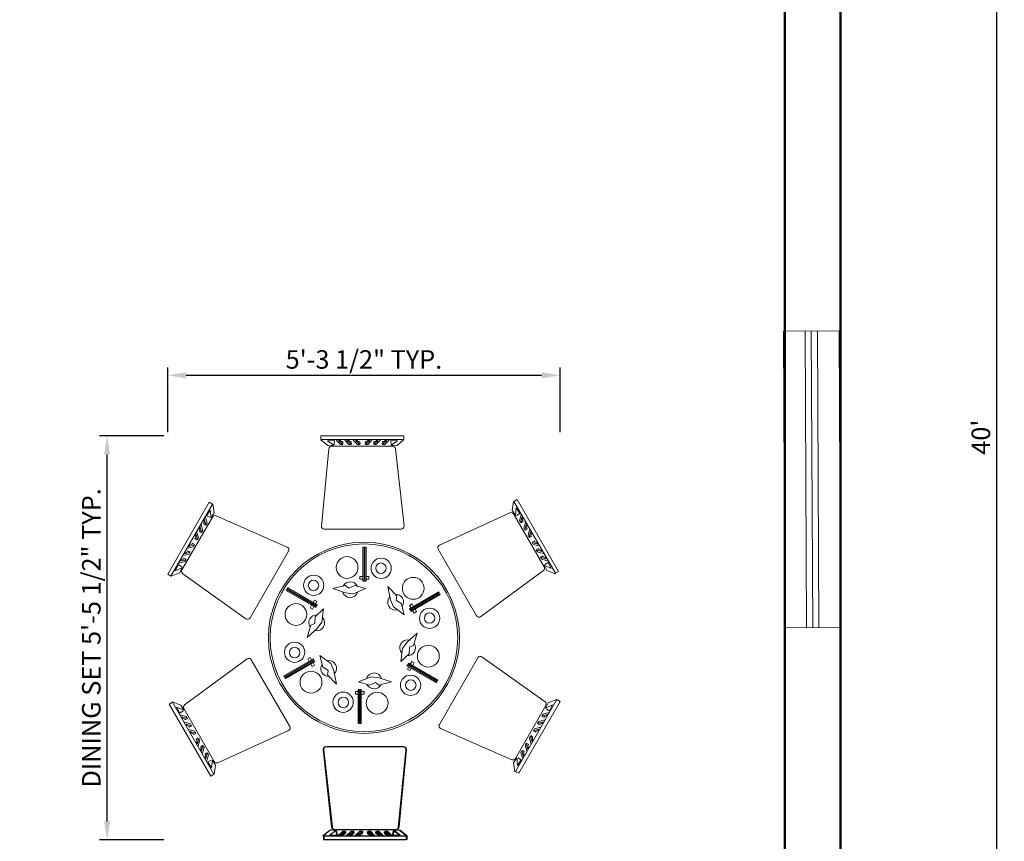
# Model space of a CAD drawing. Units: inches. Extents: x 108 to 1546, y -229 to 513.
# Tile 6 of 11: x 910 to 1070, y 171 to 304. Entities that reach past the tile are written whole.
import ezdxf

# ---------------------------------------------------------------- set-up
doc = ezdxf.new("R2010")
doc.units = ezdxf.units.IN
for name, color, linetype, lineweight in [('A-ANNO-DIMS', 2, 'Continuous', 18), ('A-FURN', 8, 'Continuous', 13), ('wall', 7, 'Continuous', 50), ('WINDOW', 212, 'Continuous', 18)]:
    doc.layers.add(name, color=color, linetype=linetype, lineweight=lineweight)
doc.styles.get("Standard").update_dxf_attribs({"font": 'arial.ttf'})
doc.dimstyles.new('ISO-25', dxfattribs={"dimtxt": 3, "dimasz": 3, "dimexe": 1.25, "dimexo": 0.625, "dimtad": 1, "dimdec": 1, "dimlunit": 3, "dimtxsty": 'Standard', "dimcen": 2.5, "dimadec": 0, "dimazin": 0, "dimtfac": 1, "dimtdec": 1, "dimtmove": 0, "dimatfit": 3, "dimfxl": 1, "dimarcsym": 0})

# ---------------------------------------------------------------- blocks, each defined once
blk = doc.blocks.new('A$C45501D90')
for p, q in [((-242.2, 1133.5), (224, 1133.5)), ((-242.2, 1112.8), (-242.2, 1133.5)), ((224, 1112.8), (-242.2, 1112.8)), ((-242.2, 1111.2), (-202.3, 1079.2)), ((-203.9, 1106.4), (-165.6, 1108)), ((-165.6, 1108), (-167.2, 1085.6)), ((-156, 1109.6), (-132, 1085.6)), ((-119.3, 1085.6), (-143.2, 1108)), ((-143.2, 1108), (-133.6, 1108)), ((-133.6, 1108), (-122.5, 1098.4)), ((-108.1, 1109.6), (-84.1, 1085.6)), ((-71.4, 1085.6), (-95.3, 1108)), ((-95.3, 1108), (-85.7, 1108)), ((-85.7, 1108), (-74.6, 1098.4)), ((-60.2, 1109.6), (-36.2, 1085.6)), ((-23.5, 1085.6), (-47.4, 1108)), ((-47.4, 1108), (-37.8, 1108)), ((-37.8, 1108), (-26.7, 1098.4)), ((8.5, 1085.6), (32.4, 1108)), ((22.8, 1108), (11.6, 1098.4)), ((45.2, 1109.6), (21.2, 1085.6)), ((32.4, 1108), (22.8, 1108)), ((56.3, 1085.6), (80.3, 1108)), ((70.7, 1108), (59.5, 1098.4)), ((93.1, 1109.6), (69.1, 1085.6)), ((80.3, 1108), (70.7, 1108)), ((104.2, 1085.6), (128.2, 1108)), ((118.6, 1108), (107.4, 1098.4)), ((141, 1109.6), (117, 1085.6)), ((128.2, 1108), (118.6, 1108)), ((188.9, 1106.4), (150.5, 1108)), ((150.5, 1108), (152.1, 1085.6)), ((224, 1112.8), (187.3, 1079.2)), ((224, 1133.5), (224, 1112.8)), ((-197.3, 1061.6), (-238.9, 627.6)), ((-168.8, 1080.8), (-203.9, 1106.4)), ((-202.3, 1079.2), (-168.8, 1080.8)), ((161.8, 1076.1), (-181.4, 1076.1)), ((-132, 1085.6), (-119.3, 1085.6)), ((-122.5, 1098.4), (-119.3, 1101.6)), ((-119.3, 1101.6), (-117.7, 1087.2)), ((-84.1, 1085.6), (-71.4, 1085.6)), ((-74.6, 1098.4), (-71.4, 1101.6)), ((-71.4, 1101.6), (-69.8, 1087.2)), ((-36.2, 1085.6), (-23.5, 1085.6)), ((-26.7, 1098.4), (-23.5, 1101.6)), ((-23.5, 1101.6), (-21.9, 1087.2)), ((8.5, 1101.6), (6.9, 1087.2)), ((11.6, 1098.4), (8.5, 1101.6)), ((21.2, 1085.6), (8.5, 1085.6)), ((56.3, 1101.6), (54.8, 1087.2)), ((59.5, 1098.4), (56.3, 1101.6)), ((69.1, 1085.6), (56.3, 1085.6)), ((104.2, 1101.6), (102.6, 1087.2)), ((107.4, 1098.4), (104.2, 1101.6)), ((117, 1085.6), (104.2, 1085.6)), ((153.7, 1080.8), (188.9, 1106.4)), ((187.3, 1079.2), (153.7, 1080.8)), ((225.2, 627.8), (177.6, 1061.8)), ((842.6, 766.1), (860.5, 776.5)), ((860.5, 776.5), (1093.6, 372.8)), ((-1102.7, 357), (-869.7, 760.7)), ((-851.7, 750.4), (-1084.8, 346.6)), ((-869.7, 760.7), (-851.7, 750.4)), ((-848.7, 752.3), (-841, 701.8)), ((841.2, 765.3), (833.5, 714.8)), ((1075.7, 362.4), (842.6, 766.1)), ((851.7, 686.6), (856.2, 729.8)), ((856.2, 729.8), (876.7, 697.4)), ((-851, 678.1), (-1022.6, 380.9)), ((-895.4, 665), (-900.2, 656.7)), ((-888.1, 633.1), (-895.4, 665)), ((-890.4, 676.9), (-881.7, 644.2)), ((-863.7, 716.7), (-884.3, 684.4)), ((-884.3, 684.4), (-864.1, 674.6)), ((-859.2, 673.6), (-863.7, 716.7)), ((-841, 701.8), (-859.2, 673.6)), ((-431.1, 509), (-830.8, 684.8)), ((820.7, 701.7), (424.1, 520.7)), ((833.5, 714.8), (851.7, 686.6)), ((1012.8, 397.9), (841.2, 695.1)), ((876.7, 697.4), (856.6, 687.6)), ((882.9, 689.9), (874.2, 657.2)), ((880.6, 646.1), (887.9, 678)), ((887.9, 678), (892.7, 669.7)), ((892.7, 669.7), (890, 655.2)), ((-919.4, 623.5), (-924.2, 615.2)), ((-924.2, 615.2), (-921.5, 600.8)), ((-912, 591.6), (-919.4, 623.5)), ((-914.4, 635.4), (-905.6, 602.7)), ((-897.5, 642.2), (-901.9, 641.1)), ((-901.9, 641.1), (-890.2, 632.5)), ((-900.2, 656.7), (-897.5, 642.2)), ((-881.7, 644.2), (-888.1, 633.1)), ((-223, 610.1), (209.4, 610.1)), ((874.2, 657.2), (880.6, 646.1)), ((894.4, 654.1), (882.7, 645.5)), ((890, 655.2), (894.4, 654.1)), ((906.9, 648.4), (898.1, 615.7)), ((898.1, 615.7), (904.5, 604.6)), ((904.5, 604.6), (911.9, 636.5)), ((918.3, 612.6), (906.7, 604)), ((911.9, 636.5), (916.7, 628.2)), ((916.7, 628.2), (914, 613.8)), ((914, 613.8), (918.3, 612.6)), ((-945.4, 559.3), (-949.8, 558.1)), ((-949.8, 558.1), (-938.1, 549.6)), ((-943.3, 582), (-948.1, 573.8)), ((-948.1, 573.8), (-945.4, 559.3)), ((-936, 550.1), (-943.3, 582)), ((-938.3, 593.9), (-929.6, 561.2)), ((-929.6, 561.2), (-936, 550.1)), ((-921.5, 600.8), (-925.8, 599.6)), ((-925.8, 599.6), (-914.2, 591)), ((-905.6, 602.7), (-912, 591.6)), ((930.8, 606.9), (922.1, 574.2)), ((922.1, 574.2), (928.4, 563.1)), ((928.4, 563.1), (935.8, 595.1)), ((942.3, 571.1), (930.6, 562.6)), ((935.8, 595.1), (940.6, 586.8)), ((940.6, 586.8), (937.9, 572.3)), ((937.9, 572.3), (942.3, 571.1)), ((-991, 502.7), (-958.3, 511.4)), ((-951.9, 522.5), (-983.2, 512.9)), ((-983.2, 512.9), (-978.5, 521.2)), ((-978.5, 521.2), (-964.6, 526.1)), ((-964.6, 526.1), (-965.7, 530.5)), ((-965.7, 530.5), (-952.5, 524.7)), ((-958.3, 511.4), (-951.9, 522.5)), ((-5.6, 508.7, 90.8), (0.4, 508.7, 90.8)), ((-5.6, 317.7, 90.8), (-5.6, 508.7, 90.8)), ((0.4, 508.7, 90.8), (0.4, 317.7, 90.8)), ((5.8, 317.7, 90.8), (5.8, 508.7, 90.8)), ((5.8, 508.7, 90.8), (11.8, 508.7, 90.8)), ((11.8, 508.7, 90.8), (11.8, 317.7, 90.8)), ((416.9, 498.2), (633.1, 123.7)), ((950.8, 524.4), (944.4, 535.5)), ((944.4, 535.5), (975.7, 525.9)), ((958.2, 543.5), (945, 537.7)), ((983.5, 515.7), (950.8, 524.4)), ((957.1, 539.1), (958.2, 543.5)), ((970.9, 534.2), (957.1, 539.1)), ((982.2, 502), (968.9, 496.2)), ((975.7, 525.9), (970.9, 534.2)), ((981, 497.6), (982.2, 502)), ((-1026.3, 438.3), (-1012.5, 443.1)), ((-1015, 461.2), (-982.3, 469.9)), ((-1012.5, 443.1), (-1013.6, 447.5)), ((-1013.6, 447.5), (-1000.4, 441.7)), ((-975.9, 481), (-1007.2, 471.4)), ((-1007.2, 471.4), (-1002.4, 479.7)), ((-1002.4, 479.7), (-988.5, 484.6)), ((-988.5, 484.6), (-989.7, 489)), ((-989.7, 489), (-976.5, 483.2)), ((-982.3, 469.9), (-975.9, 481)), ((-639.9, 111.9), (-423.7, 486.4)), ((968.4, 494), (999.7, 484.4)), ((974.7, 483), (968.4, 494)), ((1007.4, 474.2), (974.7, 483)), ((994.9, 492.7), (981, 497.6)), ((998.7, 441.5), (992.3, 452.5)), ((992.3, 452.5), (1023.6, 443)), ((1006.1, 460.5), (992.9, 454.7)), ((999.7, 484.4), (994.9, 492.7)), ((1005, 456.2), (1006.1, 460.5)), ((1018.8, 451.3), (1005, 456.2)), ((1023.6, 443), (1018.8, 451.3)), ((-1060.1, 376.6), (-1042.3, 410.6)), ((-1020.4, 394.3), (-1060.1, 376.6)), ((-1042.3, 410.6), (-1023.8, 398.1)), ((-1038.9, 419.7), (-1006.2, 428.5)), ((-1035.8, 364.4), (-1020.4, 394.3)), ((-999.8, 439.5), (-1031.1, 430)), ((-1031.1, 430), (-1026.3, 438.3)), ((-1006.2, 428.5), (-999.8, 439.5)), ((1031.4, 432.7), (998.7, 441.5)), ((1028.3, 377.5), (1012.9, 407.3)), ((1012.9, 407.3), (1052.6, 389.6)), ((1034.8, 423.6), (1016.3, 411.1)), ((1052.6, 389.6), (1034.8, 423.6)), ((-1084.8, 346.6), (-1102.7, 357)), ((-1083.4, 345.8), (-1035.8, 364.4)), ((-1018, 360), (-663, 106.9)), ((-22.3, 329.1, 90.8), (-22.3, 344.6, 90.8)), ((-22.3, 344.6, 90.8), (-5.6, 344.6, 90.8)), ((0.4, 344.6, 90.8), (5.8, 344.6, 90.8)), ((11.8, 344.6, 90.8), (27.3, 344.6, 90.8)), ((27.3, 344.6, 90.8), (27.3, 329.1, 90.8)), ((656.3, 118.9), (1008.4, 377.1)), ((1075.9, 358.8), (1028.3, 377.5)), ((1093.6, 372.8), (1075.7, 362.4)), ((-430.6, 275.2, 90.8), (-427.6, 280.3, 90.8)), ((-427.6, 280.3, 90.8), (-262.3, 184.9, 90.8)), ((-175.3, 276.1, 90.8), (-104.8, 293.2, 90.8)), ((-104.8, 293.2, 90.8), (-85.5, 278.4, 90.8)), ((-85.5, 278.4, 90.8), (-52.1, 293.9, 90.8)), ((-52.1, 293.9, 90.8), (9.5, 276.1, 90.8)), ((-5.6, 329.1, 90.8), (-22.3, 329.1, 90.8)), ((0.4, 317.7, 90.8), (-5.6, 317.7, 90.8)), ((5.8, 329.1, 90.8), (0.4, 329.1, 90.8)), ((11.8, 317.7, 90.8), (5.8, 317.7, 90.8)), ((27.3, 329.1, 90.8), (11.8, 329.1, 90.8)), ((134.3, 288, 90.8), (184.3, 235.5, 90.8)), ((149.7, 213.9, 90.8), (134.3, 288, 90.8)), ((-436.3, 265.3, 90.8), (-433.3, 270.5, 90.8)), ((-270.9, 169.9, 90.8), (-436.3, 265.3, 90.8)), ((-433.3, 270.5, 90.8), (-267.9, 175, 90.8)), ((-265.2, 179.7, 90.8), (-430.6, 275.2, 90.8)), ((-103.3, 252.4, 90.8), (-175.3, 276.1, 90.8)), ((-59.5, 246.5, 90.8), (-103.3, 252.4, 90.8)), ((9.5, 276.1, 90.8), (-59.5, 246.5, 90.8)), ((184.3, 235.5, 90.8), (181.1, 211.4, 90.8)), ((255.2, 161.9, 90.8), (420.6, 257.3, 90.8)), ((423.5, 252.2, 90.8), (258.2, 156.7, 90.8)), ((260.9, 152, 90.8), (426.2, 247.5, 90.8)), ((429.2, 242.3, 90.8), (263.8, 146.9, 90.8)), ((420.6, 257.3, 90.8), (423.5, 252.2, 90.8)), ((426.2, 247.5, 90.8), (429.2, 242.3, 90.8)), ((-302.5, 168.8, 90.8), (-294.2, 183.3, 90.8)), ((-289.1, 161.1, 90.8), (-302.5, 168.8, 90.8)), ((-291.2, 188.5, 90.8), (-288.5, 193.1, 90.8)), ((-280.7, 175.5, 90.8), (-289.1, 161.1, 90.8)), ((-285.5, 198.3, 90.8), (-277.8, 211.7, 90.8)), ((-277.8, 211.7, 90.8), (-264.3, 204, 90.8)), ((-275.1, 185.4, 90.8), (-277.8, 180.7, 90.8)), ((-264.3, 204, 90.8), (-272.1, 190.5, 90.8)), ((-267.9, 175, 90.8), (-270.9, 169.9, 90.8)), ((-262.3, 184.9, 90.8), (-265.2, 179.7, 90.8)), ((166.5, 173, 90.8), (149.7, 213.9, 90.8)), ((226.7, 128.1, 90.8), (166.5, 173, 90.8)), ((181.1, 211.4, 90.8), (211.3, 190.3, 90.8)), ((211.3, 190.3, 90.8), (226.7, 128.1, 90.8)), ((256.6, 182, 90.8), (270.1, 189.8, 90.8)), ((265, 167.5, 90.8), (256.6, 182, 90.8)), ((270.1, 189.8, 90.8), (278.4, 175.3, 90.8)), ((281.4, 170.1, 90.8), (284.1, 165.5, 90.8)), ((-276.8, 80.9, 90.8), (-273.6, 117.6, 90.8)), ((-273.6, 117.6, 90.8), (-227.4, 162.1, 90.8)), ((-227.4, 162.1, 90.8), (-236.2, 87.5, 90.8)), ((258.2, 156.7, 90.8), (255.2, 161.9, 90.8)), ((263.8, 146.9, 90.8), (260.9, 152, 90.8)), ((270.7, 157.7, 90.8), (268, 162.4, 90.8)), ((281.4, 139.1, 90.8), (273.7, 152.5, 90.8)), ((294.9, 146.8, 90.8), (281.4, 139.1, 90.8)), ((287.1, 160.3, 90.8), (294.9, 146.8, 90.8)), ((-319.8, 2.1, 90.8), (-299.3, 71.7, 90.8)), ((-299.3, 71.7, 90.8), (-276.8, 80.9, 90.8)), ((-236.2, 87.5, 90.8), (-263.2, 52.5, 90.8)), ((-263.2, 52.5, 90.8), (-319.8, 2.1, 90.8)), ((242.9, -24.6, 90.8), (299.4, 25.9, 90.8)), ((299.4, 25.9, 90.8), (278.9, -43.7, 90.8)), ((215.8, -59.5, 90.8), (242.9, -24.6, 90.8)), ((256.4, -53, 90.8), (253.2, -89.7, 90.8)), ((278.9, -43.7, 90.8), (256.4, -53, 90.8)), ((-247, -100.1, 90.8), (-186.8, -145, 90.8)), ((-231.7, -162.3, 90.8), (-247, -100.1, 90.8)), ((207, -134.1, 90.8), (215.8, -59.5, 90.8)), ((253.2, -89.7, 90.8), (207, -134.1, 90.8)), ((1018, -360), (663, -106.9)), ((-656.3, -118.9), (-1008.4, -377.1)), ((-416.9, -498.2), (-633.1, -123.7)), ((-449.6, -214.4, 90.8), (-284.2, -118.9, 90.8)), ((-281.2, -124.1, 90.8), (-446.6, -219.5, 90.8)), ((-443.9, -224.2, 90.8), (-278.5, -128.7, 90.8)), ((-275.5, -133.9, 90.8), (-440.9, -229.4, 90.8)), ((-315.2, -118.9, 90.8), (-301.8, -111.1, 90.8)), ((-307.5, -132.3, 90.8), (-315.2, -118.9, 90.8)), ((-301.8, -142.1, 90.8), (-304.5, -137.5, 90.8)), ((-301.8, -111.1, 90.8), (-294, -124.6, 90.8)), ((-290.4, -161.8, 90.8), (-298.8, -147.3, 90.8)), ((-291, -129.7, 90.8), (-288.3, -134.4, 90.8)), ((-277, -154, 90.8), (-290.4, -161.8, 90.8)), ((-285.4, -139.5, 90.8), (-277, -154, 90.8)), ((-284.2, -118.9, 90.8), (-281.2, -124.1, 90.8)), ((-278.5, -128.7, 90.8), (-275.5, -133.9, 90.8)), ((-201.5, -183.4, 90.8), (-231.7, -162.3, 90.8)), ((-186.8, -145, 90.8), (-170.1, -185.9, 90.8)), ((241.9, -156.9, 90.8), (244.9, -151.7, 90.8)), ((407.3, -252.4, 90.8), (241.9, -156.9, 90.8)), ((244, -176, 90.8), (251.7, -162.5, 90.8)), ((244.9, -151.7, 90.8), (410.3, -247.2, 90.8)), ((247.6, -147.1, 90.8), (250.6, -141.9, 90.8)), ((413, -242.5, 90.8), (247.6, -147.1, 90.8)), ((250.6, -141.9, 90.8), (415.9, -237.4, 90.8)), ((254.7, -157.4, 90.8), (257.4, -152.7, 90.8)), ((260.4, -147.6, 90.8), (268.7, -133.1, 90.8)), ((270.8, -160.5, 90.8), (268.1, -165.1, 90.8)), ((268.7, -133.1, 90.8), (282.2, -140.8, 90.8)), ((282.2, -140.8, 90.8), (273.8, -155.3, 90.8)), ((639.9, -111.9), (423.7, -486.4)), ((-446.6, -219.5, 90.8), (-449.6, -214.4, 90.8)), ((-204.7, -207.6, 90.8), (-201.5, -183.4, 90.8)), ((-154.7, -260.1, 90.8), (-204.7, -207.6, 90.8)), ((-170.1, -185.9, 90.8), (-154.7, -260.1, 90.8)), ((-29.8, -248.2, 90.8), (39.2, -218.5, 90.8)), ((39.2, -218.5, 90.8), (83, -224.4, 90.8)), ((257.4, -183.7, 90.8), (244, -176, 90.8)), ((265.2, -170.3, 90.8), (257.4, -183.7, 90.8)), ((-440.9, -229.4, 90.8), (-443.9, -224.2, 90.8)), ((31.8, -266, 90.8), (-29.8, -248.2, 90.8)), ((65.2, -250.4, 90.8), (31.8, -266, 90.8)), ((84.4, -265.2, 90.8), (65.2, -250.4, 90.8)), ((83, -224.4, 90.8), (154.9, -248.2, 90.8)), ((154.9, -248.2, 90.8), (84.4, -265.2, 90.8)), ((410.3, -247.2, 90.8), (407.3, -252.4, 90.8)), ((415.9, -237.4, 90.8), (413, -242.5, 90.8)), ((-47.6, -316.6, 90.8), (-47.6, -301.1, 90.8)), ((-47.6, -301.1, 90.8), (-32.1, -301.1, 90.8)), ((-32.1, -316.6, 90.8), (-47.6, -316.6, 90.8)), ((-32.1, -480.7, 90.8), (-32.1, -289.8, 90.8)), ((-32.1, -289.8, 90.8), (-26.1, -289.8, 90.8)), ((-26.1, -289.8, 90.8), (-26.1, -480.7, 90.8)), ((-26.1, -301.1, 90.8), (-20.8, -301.1, 90.8)), ((-20.8, -316.6, 90.8), (-26.1, -316.6, 90.8)), ((-20.8, -480.7, 90.8), (-20.8, -289.8, 90.8)), ((-20.8, -289.8, 90.8), (-14.8, -289.8, 90.8)), ((-14.8, -289.8, 90.8), (-14.8, -480.7, 90.8)), ((-14.8, -301.1, 90.8), (1.9, -301.1, 90.8)), ((1.9, -316.6, 90.8), (-14.8, -316.6, 90.8)), ((1.9, -301.1, 90.8), (1.9, -316.6, 90.8)), ((-1093.6, -372.8), (-1075.7, -362.4)), ((-860.5, -776.5), (-1093.6, -372.8)), ((-1075.9, -358.8), (-1028.3, -377.5)), ((-1075.7, -362.4), (-842.6, -766.1)), ((-1028.3, -377.5), (-1012.9, -407.3)), ((851, -678.1), (1022.6, -380.9)), ((851.7, -750.4), (1084.8, -346.6)), ((1102.7, -357), (869.7, -760.7)), ((1035.8, -364.4), (1020.4, -394.3)), ((1020.4, -394.3), (1060.1, -376.6)), ((1083.4, -345.8), (1035.8, -364.4)), ((1060.1, -376.6), (1042.3, -410.6)), ((1084.8, -346.6), (1102.7, -357)), ((-1052.6, -389.6), (-1034.8, -423.6)), ((-1012.9, -407.3), (-1052.6, -389.6)), ((-1034.8, -423.6), (-1016.3, -411.1)), ((-1031.4, -432.7), (-998.7, -441.5)), ((-1012.8, -397.9), (-841.2, -695.1)), ((-998.7, -441.5), (-992.3, -452.5)), ((1006.2, -428.5), (999.8, -439.5)), ((999.8, -439.5), (1031.1, -430)), ((1013.6, -447.5), (1000.4, -441.7)), ((1038.9, -419.7), (1006.2, -428.5)), ((1026.3, -438.3), (1012.5, -443.1)), ((1042.3, -410.6), (1023.8, -398.1)), ((1031.1, -430), (1026.3, -438.3)), ((-1023.6, -443), (-1018.8, -451.3)), ((-992.3, -452.5), (-1023.6, -443)), ((-1018.8, -451.3), (-1005, -456.2)), ((-1007.4, -474.2), (-974.7, -483)), ((-1006.1, -460.5), (-992.9, -454.7)), ((-1005, -456.2), (-1006.1, -460.5)), ((-968.4, -494), (-999.7, -484.4)), ((-999.7, -484.4), (-994.9, -492.7)), ((-994.9, -492.7), (-981, -497.6)), ((-982.2, -502), (-968.9, -496.2)), ((-981, -497.6), (-982.2, -502)), ((-974.7, -483), (-968.4, -494)), ((-26.1, -480.7, 90.8), (-32.1, -480.7, 90.8)), ((-14.8, -480.7, 90.8), (-20.8, -480.7, 90.8)), ((982.3, -469.9), (975.9, -481)), ((975.9, -481), (1007.2, -471.4)), ((989.7, -489), (976.5, -483.2)), ((1015, -461.2), (982.3, -469.9)), ((1002.4, -479.7), (988.5, -484.6)), ((988.5, -484.6), (989.7, -489)), ((1007.2, -471.4), (1002.4, -479.7)), ((1012.5, -443.1), (1013.6, -447.5)), ((-983.5, -515.7), (-950.8, -524.4)), ((-944.4, -535.5), (-975.7, -525.9)), ((-975.7, -525.9), (-970.9, -534.2)), ((-970.9, -534.2), (-957.1, -539.1)), ((-958.2, -543.5), (-945, -537.7)), ((-957.1, -539.1), (-958.2, -543.5)), ((-950.8, -524.4), (-944.4, -535.5)), ((-820.7, -701.7), (-424.1, -520.7)), ((431.1, -509), (830.8, -684.8)), ((929.6, -561.2), (936, -550.1)), ((936, -550.1), (943.3, -582)), ((949.8, -558.1), (938.1, -549.6)), ((958.3, -511.4), (951.9, -522.5)), ((951.9, -522.5), (983.2, -512.9)), ((965.7, -530.5), (952.5, -524.7)), ((991, -502.7), (958.3, -511.4)), ((978.5, -521.2), (964.6, -526.1)), ((964.6, -526.1), (965.7, -530.5)), ((983.2, -512.9), (978.5, -521.2)), ((-942.3, -571.1), (-930.6, -562.6)), ((-937.9, -572.3), (-942.3, -571.1)), ((-940.6, -586.8), (-937.9, -572.3)), ((-935.8, -595.1), (-940.6, -586.8)), ((-928.4, -563.1), (-935.8, -595.1)), ((-930.8, -606.9), (-922.1, -574.2)), ((-922.1, -574.2), (-928.4, -563.1)), ((-918.3, -612.6), (-906.7, -604)), ((-904.5, -604.6), (-911.9, -636.5)), ((-898.1, -615.7), (-904.5, -604.6)), ((905.6, -602.7), (912, -591.6)), ((914.4, -635.4), (905.6, -602.7)), ((912, -591.6), (919.4, -623.5)), ((925.8, -599.6), (914.2, -591)), ((921.5, -600.8), (925.8, -599.6)), ((924.2, -615.2), (921.5, -600.8)), ((938.3, -593.9), (929.6, -561.2)), ((943.3, -582), (948.1, -573.8)), ((945.4, -559.3), (949.8, -558.1)), ((948.1, -573.8), (945.4, -559.3)), ((-914, -613.8), (-918.3, -612.6)), ((-916.7, -628.2), (-914, -613.8)), ((-911.9, -636.5), (-916.7, -628.2)), ((-906.9, -648.4), (-898.1, -615.7)), ((-894.4, -654.1), (-882.7, -645.5)), ((-890, -655.2), (-894.4, -654.1)), ((-892.7, -669.7), (-890, -655.2)), ((-880.6, -646.1), (-887.9, -678)), ((-882.9, -689.9), (-874.2, -657.2)), ((-874.2, -657.2), (-880.6, -646.1)), ((-229.3, -629.3), (-181.8, -1063.3)), ((-225.2, -627.8), (-177.6, -1061.8)), ((218.9, -611.6), (-213.5, -611.6)), ((223, -610.1), (-209.4, -610.1)), ((193.2, -1063.1), (234.8, -629.1)), ((197.3, -1061.6), (238.9, -627.6)), ((881.7, -644.2), (888.1, -633.1)), ((890.4, -676.9), (881.7, -644.2)), ((888.1, -633.1), (895.4, -665)), ((901.9, -641.1), (890.2, -632.5)), ((895.4, -665), (900.2, -656.7)), ((897.5, -642.2), (901.9, -641.1)), ((900.2, -656.7), (897.5, -642.2)), ((919.4, -623.5), (924.2, -615.2)), ((-887.9, -678), (-892.7, -669.7)), ((-876.7, -697.4), (-856.6, -687.6)), ((-856.2, -729.8), (-876.7, -697.4)), ((-851.7, -686.6), (-856.2, -729.8)), ((-833.5, -714.8), (-851.7, -686.6)), ((-841.2, -765.3), (-833.5, -714.8)), ((841, -701.8), (859.2, -673.6)), ((848.7, -752.3), (841, -701.8)), ((859.2, -673.6), (863.7, -716.7)), ((863.7, -716.7), (884.3, -684.4)), ((884.3, -684.4), (864.1, -674.6)), ((-842.6, -766.1), (-860.5, -776.5)), ((869.7, -760.7), (851.7, -750.4)), ((-231.3, -1112.7), (-191.4, -1080.8)), ((-227.2, -1111.2), (-187.3, -1079.2)), ((-157.9, -1082.4), (-193, -1107.9)), ((-191.4, -1080.8), (-157.9, -1082.4)), ((-153.7, -1080.8), (-188.9, -1106.4)), ((-188.9, -1106.4), (-150.5, -1108)), ((-187.3, -1079.2), (-153.7, -1080.8)), ((-165.9, -1077.6), (177.3, -1077.6)), ((-161.8, -1076.1), (181.4, -1076.1)), ((-154.7, -1109.5), (-156.3, -1087.1)), ((-150.5, -1108), (-152.1, -1085.6)), ((-145.1, -1111.1), (-121.1, -1087.1)), ((-141, -1109.6), (-117, -1085.6)), ((-108.4, -1087.1), (-132.3, -1109.5)), ((-104.2, -1085.6), (-128.2, -1108)), ((-122.7, -1109.5), (-111.6, -1099.9)), ((-121.1, -1087.1), (-108.4, -1087.1)), ((-118.6, -1108), (-107.4, -1098.4)), ((-117, -1085.6), (-104.2, -1085.6)), ((-111.6, -1099.9), (-108.4, -1103.1)), ((-108.4, -1103.1), (-106.8, -1088.7)), ((-107.4, -1098.4), (-104.2, -1101.6)), ((-104.2, -1101.6), (-102.6, -1087.2)), ((-97.2, -1111.1), (-73.2, -1087.1)), ((-93.1, -1109.6), (-69.1, -1085.6)), ((-60.5, -1087.1), (-84.4, -1109.5)), ((-56.3, -1085.6), (-80.3, -1108)), ((-74.8, -1109.5), (-63.7, -1099.9)), ((-73.2, -1087.1), (-60.5, -1087.1)), ((-70.7, -1108), (-59.5, -1098.4)), ((-69.1, -1085.6), (-56.3, -1085.6)), ((-63.7, -1099.9), (-60.5, -1103.1)), ((-60.5, -1103.1), (-58.9, -1088.7)), ((-59.5, -1098.4), (-56.3, -1101.6)), ((-56.3, -1101.6), (-54.8, -1087.2)), ((-49.3, -1111.1), (-25.3, -1087.1)), ((-45.2, -1109.6), (-21.2, -1085.6)), ((-12.6, -1087.1), (-36.5, -1109.5)), ((-8.5, -1085.6), (-32.4, -1108)), ((-26.9, -1109.5), (-15.8, -1099.9)), ((-25.3, -1087.1), (-12.6, -1087.1)), ((-22.8, -1108), (-11.6, -1098.4)), ((-21.2, -1085.6), (-8.5, -1085.6)), ((-15.8, -1099.9), (-12.6, -1103.1)), ((-12.6, -1103.1), (-11, -1088.7)), ((-11.6, -1098.4), (-8.5, -1101.6)), ((-8.5, -1101.6), (-6.9, -1087.2)), ((19.4, -1103.1), (17.8, -1088.7)), ((19.4, -1087.1), (43.3, -1109.5)), ((32.1, -1087.1), (19.4, -1087.1)), ((22.6, -1099.9), (19.4, -1103.1)), ((23.5, -1101.6), (21.9, -1087.2)), ((33.7, -1109.5), (22.6, -1099.9)), ((23.5, -1085.6), (47.4, -1108)), ((36.2, -1085.6), (23.5, -1085.6)), ((26.7, -1098.4), (23.5, -1101.6)), ((37.8, -1108), (26.7, -1098.4)), ((56.1, -1111.1), (32.1, -1087.1)), ((60.2, -1109.6), (36.2, -1085.6)), ((67.3, -1103.1), (65.7, -1088.7)), ((67.3, -1087.1), (91.2, -1109.5)), ((80, -1087.1), (67.3, -1087.1)), ((70.4, -1099.9), (67.3, -1103.1)), ((71.4, -1101.6), (69.8, -1087.2)), ((81.6, -1109.5), (70.4, -1099.9)), ((71.4, -1085.6), (95.3, -1108)), ((84.1, -1085.6), (71.4, -1085.6)), ((74.6, -1098.4), (71.4, -1101.6)), ((85.7, -1108), (74.6, -1098.4)), ((104, -1111.1), (80, -1087.1)), ((108.1, -1109.6), (84.1, -1085.6)), ((115.1, -1103.1), (113.6, -1088.7)), ((115.1, -1087.1), (139.1, -1109.5)), ((127.9, -1087.1), (115.1, -1087.1)), ((118.3, -1099.9), (115.1, -1103.1)), ((119.3, -1101.6), (117.7, -1087.2)), ((129.5, -1109.5), (118.3, -1099.9)), ((119.3, -1085.6), (143.2, -1108)), ((132, -1085.6), (119.3, -1085.6)), ((122.5, -1098.4), (119.3, -1101.6)), ((133.6, -1108), (122.5, -1098.4)), ((151.9, -1111.1), (127.9, -1087.1)), ((156, -1109.6), (132, -1085.6)), ((161.4, -1109.5), (163, -1087.1)), ((198.2, -1080.8), (164.6, -1082.4)), ((164.6, -1082.4), (199.8, -1107.9)), ((165.6, -1108), (167.2, -1085.6)), ((203.9, -1106.4), (165.6, -1108)), ((202.3, -1079.2), (168.8, -1080.8)), ((168.8, -1080.8), (203.9, -1106.4)), ((238.1, -1112.7), (198.2, -1080.8)), ((242.2, -1111.2), (202.3, -1079.2)), ((-228.1, -1114.3), (238.1, -1114.3)), ((-228.1, -1135), (-228.1, -1114.3)), ((238.1, -1135), (-228.1, -1135)), ((-224, -1112.8), (242.2, -1112.8)), ((-224, -1133.5), (-224, -1112.8)), ((242.2, -1133.5), (-224, -1133.5)), ((-193, -1107.9), (-154.7, -1109.5)), ((-132.3, -1109.5), (-122.7, -1109.5)), ((-128.2, -1108), (-118.6, -1108)), ((-84.4, -1109.5), (-74.8, -1109.5)), ((-80.3, -1108), (-70.7, -1108)), ((-36.5, -1109.5), (-26.9, -1109.5)), ((-32.4, -1108), (-22.8, -1108)), ((43.3, -1109.5), (33.7, -1109.5)), ((47.4, -1108), (37.8, -1108)), ((91.2, -1109.5), (81.6, -1109.5)), ((95.3, -1108), (85.7, -1108)), ((139.1, -1109.5), (129.5, -1109.5)), ((143.2, -1108), (133.6, -1108)), ((199.8, -1107.9), (161.4, -1109.5)), ((238.1, -1114.3), (238.1, -1135)), ((242.2, -1112.8), (242.2, -1133.5))]:
    blk.add_line(p, q)
for centre, radius in [((0, 0), 537), ((0, 0), 527), ((-94.8, 394.7, 90.8), 61.3), ((96.9, 390, 90.8), 56.9), ((95.5, 390.7, 90.8), 29.4), ((-282.3, 294.7, 90.8), 56.9), ((277.2, 277.6, 90.8), 61.3), ((-283.5, 293.9, 90.8), 29.4), ((-382.1, 131.1, 90.8), 61.3), ((369, 109.3, 90.8), 56.9), ((368.9, 110.8, 90.8), 29.4), ((-389.3, -81.3, 90.8), 56.9), ((-389.2, -82.8, 90.8), 29.4), ((361.8, -103.1, 90.8), 61.3), ((-297.5, -249.6, 90.8), 61.3), ((261.9, -266.7, 90.8), 56.9), ((263.2, -265.9, 90.8), 29.4), ((-117.2, -362, 90.8), 56.9), ((74.4, -366.7, 90.8), 61.3), ((-115.9, -362.7, 90.8), 29.4)]:
    blk.add_circle(centre, radius)
for centre, radius, start, end in [((-181.4, 1060.1), 16, 90, 174.5199), ((161.8, 1060.1), 16, 6.2572, 90), ((-837.2, 670.1), 16, 66.2572, 150), ((827.4, 687.1), 16, 30, 114.5199), ((-223, 626.1), 16, 174.5199, 270), ((209.4, 626.1), 16, 270, 6.2572), ((-437.5, 494.4), 16, 330, 66.2572), ((430.7, 506.2), 16, 114.5199, 210), ((999, 389.9), 16, 306.2572, 30), ((-1008.8, 373), 16, 150, 234.5199), ((-77.3, 270.2, 90.8), 44.6, 25.8558, 153.3359), ((-77.3, 270.2, 90.8), 44.6, 195.9338, 342.9389), ((178.1, 200.3, 90.8), 44.6, 135.9338, 282.9389), ((178.1, 200.3, 90.8), 44.6, 325.8558, 93.3359), ((-653.7, 119.9), 16, 234.5199, 330), ((-265.7, 83.9, 90.8), 44.6, 85.8558, 213.3359), ((-265.7, 83.9, 90.8), 44.6, 255.9338, 42.9389), ((646.9, 131.7), 16, 210, 306.2572), ((245.3, -55.9, 90.8), 44.6, 75.9338, 222.9389), ((245.3, -55.9, 90.8), 44.6, 265.8558, 33.3359), ((653.7, -119.9), 16, 54.5199, 150), ((-646.9, -131.7), 16, 30, 126.2572), ((-198.5, -172.3, 90.8), 44.6, 145.8558, 273.3359), ((-198.5, -172.3, 90.8), 44.6, 315.9338, 102.9389), ((57, -242.2, 90.8), 44.6, 15.9338, 162.9389), ((57, -242.2, 90.8), 44.6, 205.8558, 333.3359), ((-999, -389.9), 16, 126.2572, 210), ((1008.8, -373), 16, 330, 54.5199), ((437.5, -494.4), 16, 150, 246.2572), ((-430.7, -506.2), 16, 294.5199, 30), ((-213.5, -627.6), 16, 90, 186.2572), ((-209.4, -626.1), 16, 90, 186.2572), ((218.9, -627.6), 16, 354.5199, 90), ((223, -626.1), 16, 354.5199, 90), ((-827.4, -687.1), 16, 210, 294.5199), ((837.2, -670.1), 16, 246.2572, 330), ((-165.9, -1061.6), 16, 186.2572, 270), ((-161.8, -1060.1), 16, 186.2572, 270), ((177.3, -1061.6), 16, 270, 354.5199), ((181.4, -1060.1), 16, 270, 354.5199)]:
    blk.add_arc(centre, radius, start, end)
blk = doc.blocks.new('*D24')
at = {"layer": 'A-ANNO-DIMS', "color": 0, "lineweight": -2, "transparency": 16777216}
for p, q in [((1043.62, 476.47), (1069.53, 476.47)), ((1068.28, 473.47), (1068.28, -0.53)), ((1043.62, -3.53), (1069.53, -3.53))]:
    blk.add_line(p, q, dxfattribs=at)
at = {"layer": 'A-ANNO-DIMS', "color": 0, "transparency": 16777216}
for points in [[(1067.78, 473.47), (1068.78, 473.47), (1068.28, 476.47)], [(1067.78, -0.53), (1068.78, -0.53), (1068.28, -3.53)]]:
    blk.add_solid(points, dxfattribs=at)
at = {"layer": 'Defpoints', "color": 0, "transparency": 16777216}
for p in [(1043, 476.47), (1043, -3.53), (1068.28, -3.53)]:
    blk.add_point(p, dxfattribs=at)
at = {"layer": 'A-ANNO-DIMS', "color": 0, "transparency": 16777216, "insert": (1066.12, 236.47), "char_height": 3, "attachment_point": 5, "rotation": 90}
blk.add_mtext("40'", dxfattribs=at)
blk = doc.blocks.new('WINDOW-48X9')
for p, q in [((0, 9), (0, 0)), ((0, 9), (48, 9)), ((48, 9), (48, 0)), ((0, 5.5), (48, 5.5)), ((0, 4.5), (48, 4.5)), ((0, 3.5), (48, 3.5)), ((0, 0), (48, 0))]:
    blk.add_line(p, q)
blk = doc.blocks.new('*D54')
at = {"layer": 'A-ANNO-DIMS', "color": 0, "lineweight": -2, "transparency": 16777216}
for p, q in [((933.37, 236.67), (922.94, 236.67)), ((924.19, 174.27), (924.19, 233.67)), ((933.37, 171.27), (922.94, 171.27))]:
    blk.add_line(p, q, dxfattribs=at)
at = {"layer": 'A-ANNO-DIMS', "color": 0, "transparency": 16777216}
for points in [[(923.69, 233.67), (924.69, 233.67), (924.19, 236.67)], [(923.69, 174.27), (924.69, 174.27), (924.19, 171.27)]]:
    blk.add_solid(points, dxfattribs=at)
at = {"layer": 'Defpoints', "color": 0, "transparency": 16777216}
for p in [(924.19, 236.67), (934, 236.67), (934, 171.27)]:
    blk.add_point(p, dxfattribs=at)
at = {"layer": 'A-ANNO-DIMS', "color": 0, "transparency": 16777216, "insert": (922.01, 203.97), "char_height": 3, "attachment_point": 5, "rotation": 90}
blk.add_mtext('DINING SET 5\'-5 1/2" TYP.', dxfattribs=at)
blk = doc.blocks.new('*D55')
at = {"layer": 'A-ANNO-DIMS', "color": 0, "lineweight": -2, "transparency": 16777216}
for p, q in [((934, 237.29), (934, 247.73)), ((997.58, 237.29), (997.58, 247.73)), ((937, 246.48), (994.58, 246.48))]:
    blk.add_line(p, q, dxfattribs=at)
at = {"layer": 'A-ANNO-DIMS', "color": 0, "transparency": 16777216}
for points in [[(937, 246.98), (937, 245.98), (934, 246.48)], [(994.58, 246.98), (994.58, 245.98), (997.58, 246.48)]]:
    blk.add_solid(points, dxfattribs=at)
at = {"layer": 'Defpoints', "color": 0, "transparency": 16777216}
for p in [(997.58, 246.48), (934, 236.67), (997.58, 236.67)]:
    blk.add_point(p, dxfattribs=at)
at = {"layer": 'A-ANNO-DIMS', "color": 0, "transparency": 16777216, "insert": (965.79, 248.66), "char_height": 3, "attachment_point": 5}
blk.add_mtext('5\'-3 1/2" TYP.', dxfattribs=at)

msp = doc.modelspace()

# ---------------------------------------------------------------- linework, layer by layer
at = {"layer": 'wall'}
for p, q in [((1043, -3.53), (1043, 476.47)), ((1034, 5.47), (1034, 467.47))]:
    msp.add_line(p, q, dxfattribs=at)

# ---------------------------------------------------------------- block references
at = {"layer": 'A-FURN', "xscale": 0.0288298030706011, "yscale": 0.0288298030706011, "zscale": 0.0288298030706011}
msp.add_blockref('A$C45501D90', (965.79, 203.99, -2.62), dxfattribs=at)
at = {"layer": 'WINDOW', "rotation": 90.2799560098102}
msp.add_blockref('WINDOW-48X9', (1042.99, 205.66), dxfattribs=at)

# ---------------------------------------------------------------- dimensions: what is measured, and where the dimension line sits
at = {"layer": 'A-ANNO-DIMS'}
dim = msp.add_linear_dim(base=(1068.28, -3.53), p1=(1043, 476.47), p2=(1043, -3.53), angle=90, dimstyle='ISO-25', override={"dimclrd": 0, "dimclre": 0, "dimclrt": 0}, dxfattribs=at)
dim.commit()
dim.dimension.update_dxf_attribs({"geometry": '*D24', "text_midpoint": (1066.12, 236.47)})
dim = msp.add_linear_dim(base=(997.58, 246.48), p1=(934, 236.67), p2=(997.58, 236.67), text='<> TYP.', dimstyle='ISO-25', override={"dimdec": 1, "dimlfac": 1, "dimrnd": 0, "dimzin": 1, "dimdsep": 46, "dimlunit": 4, "dimfrac": 2}, dxfattribs=at)
dim.commit()
dim.dimension.update_dxf_attribs({"geometry": '*D55', "text_midpoint": (965.79, 248.66)})
dim = msp.add_linear_dim(base=(924.19, 236.67), p1=(934, 171.27), p2=(934, 236.67), angle=90, text='DINING SET <> TYP.', dimstyle='ISO-25', override={"dimdec": 1, "dimlfac": 1, "dimrnd": 0, "dimzin": 1, "dimdsep": 46, "dimlunit": 4, "dimfrac": 2}, dxfattribs=at)
dim.commit()
dim.dimension.update_dxf_attribs({"geometry": '*D54', "text_midpoint": (922.01, 203.97)})

doc.saveas('drawing.dxf')
